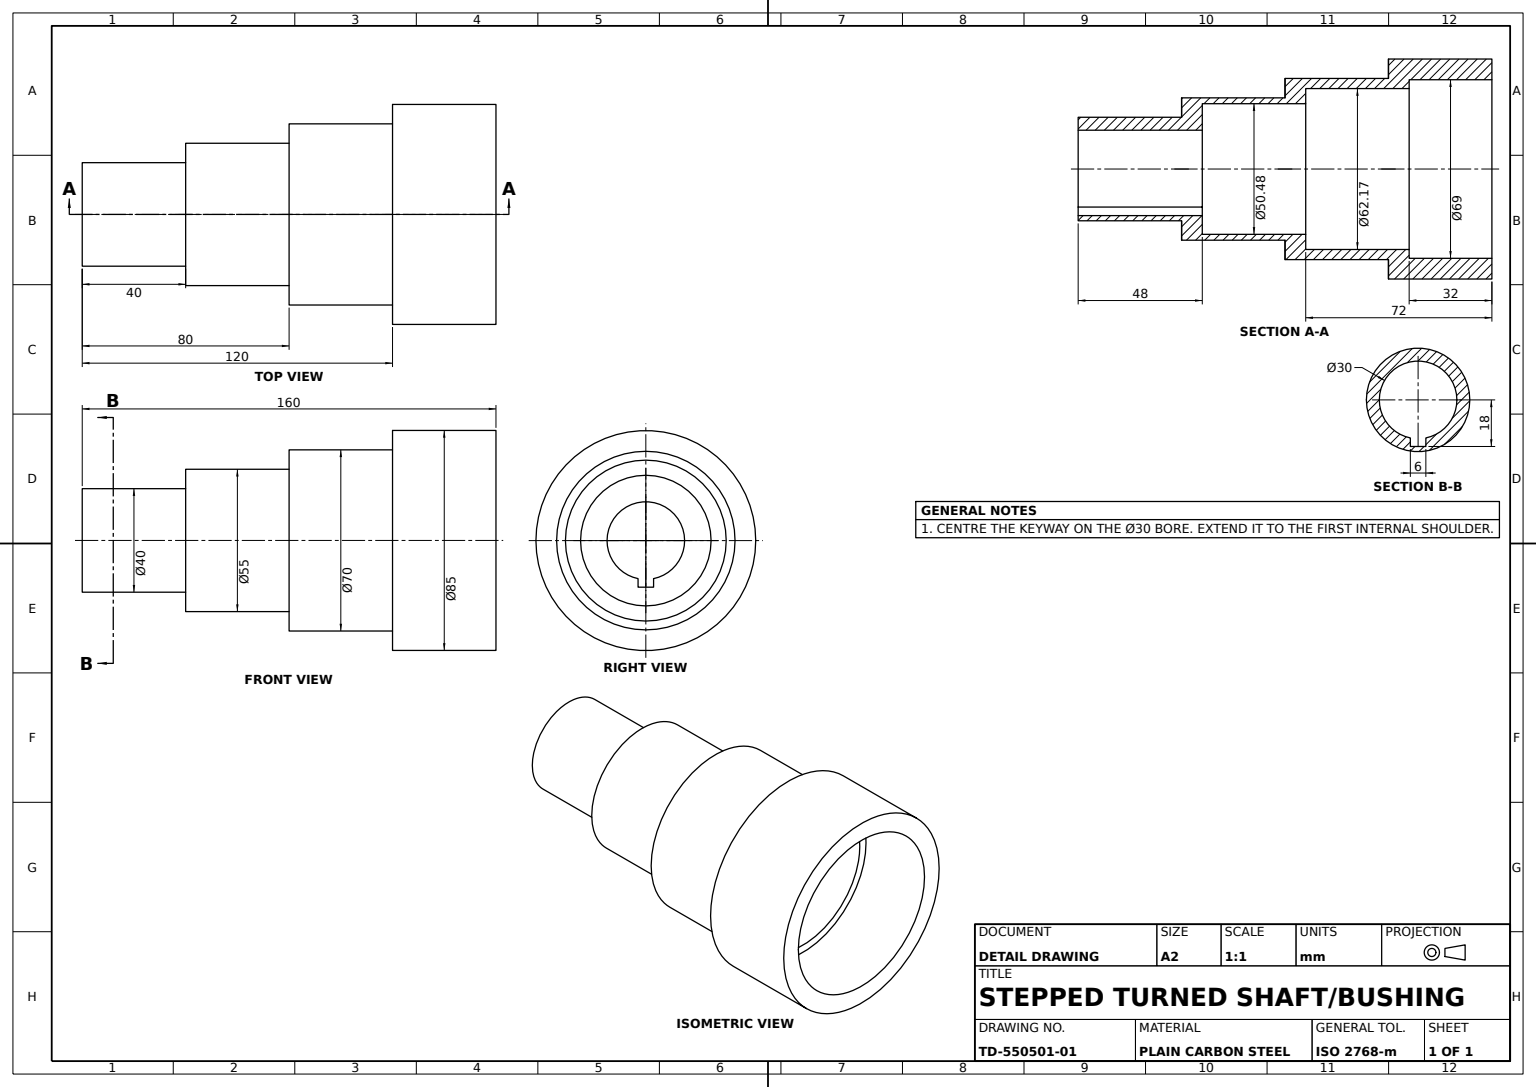
from build123d import *

# Parameters (mm, degrees)
END_BORE_30_DEEP_DEPTH = 176.261478164


with BuildPart() as part:
    # Stepped Profile Sketch → Stepped Pulley Body (revolve)
    with BuildSketch(Plane(origin=(0, 0, 0), x_dir=(1, 0, 0), z_dir=(0, 1, 0))):
        Polygon((-80, 15.035517104), (-80, 35.035517104), (-40, 35.035517104), (-40, 42.535517104), (0, 42.535517104), (0, 50.035517104), (40, 50.035517104), (40, 57.535517104), (80, 57.535517104), (80, 49.535517104), (48, 49.535517104), (48, 46.122818691), (8, 46.122818691), (8, 40.273612342), (-32, 40.273612342), (-32, 24.083136151), (40, 24.083136151), (40, 15.035517104), align=None)
    revolve(axis=Axis((40, 0, -15.035517104), (-1, 0, 0)))

    # End Bore Sketch → End Bore 30 Deep (cut, through all)
    with BuildSketch(Plane.ZY.offset(80)):
        with BuildLine():
            Line((-15.035517104, -18), (-12.035517104, -18))
            Line((-12.035517104, -18), (-12.035517104, -14.696938457))
            ThreePointArc((-12.035517104, -14.696938457), (-15.035517104, 15), (-18.035517104, -14.696938457))
            Line((-18.035517104, -14.696938457), (-18.035517104, -18))
            Line((-18.035517104, -18), (-15.035517104, -18))
        make_face()
    extrude(amount=-END_BORE_30_DEEP_DEPTH, mode=Mode.SUBTRACT)


solid = part.part
